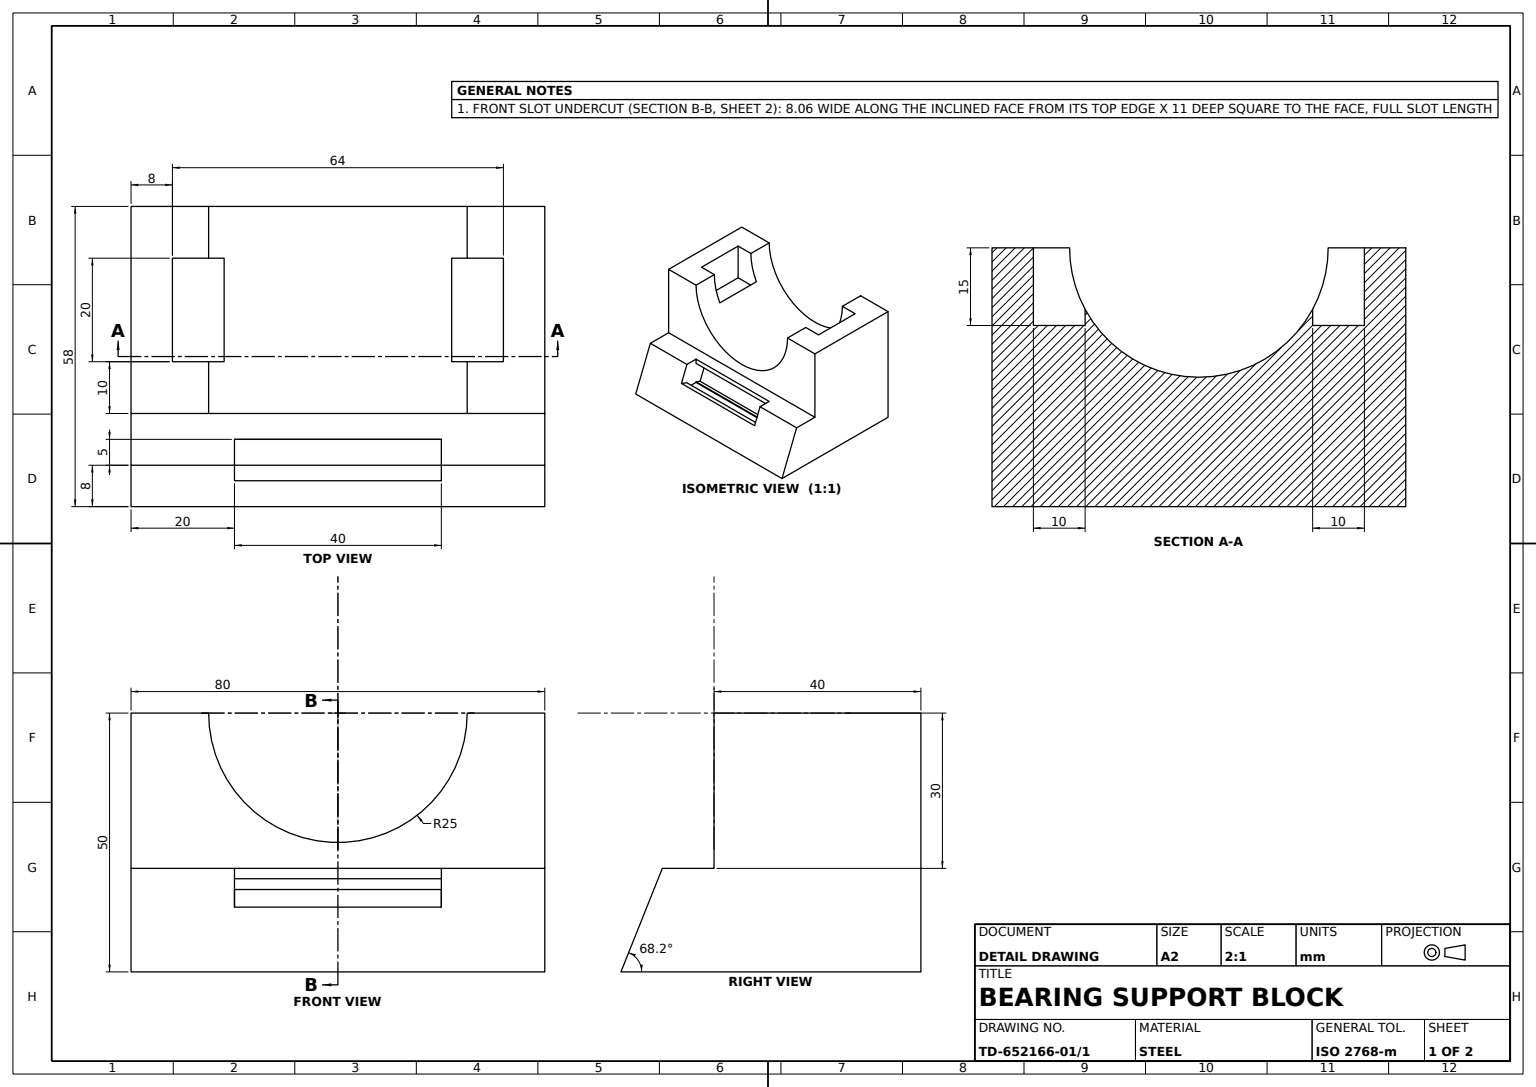
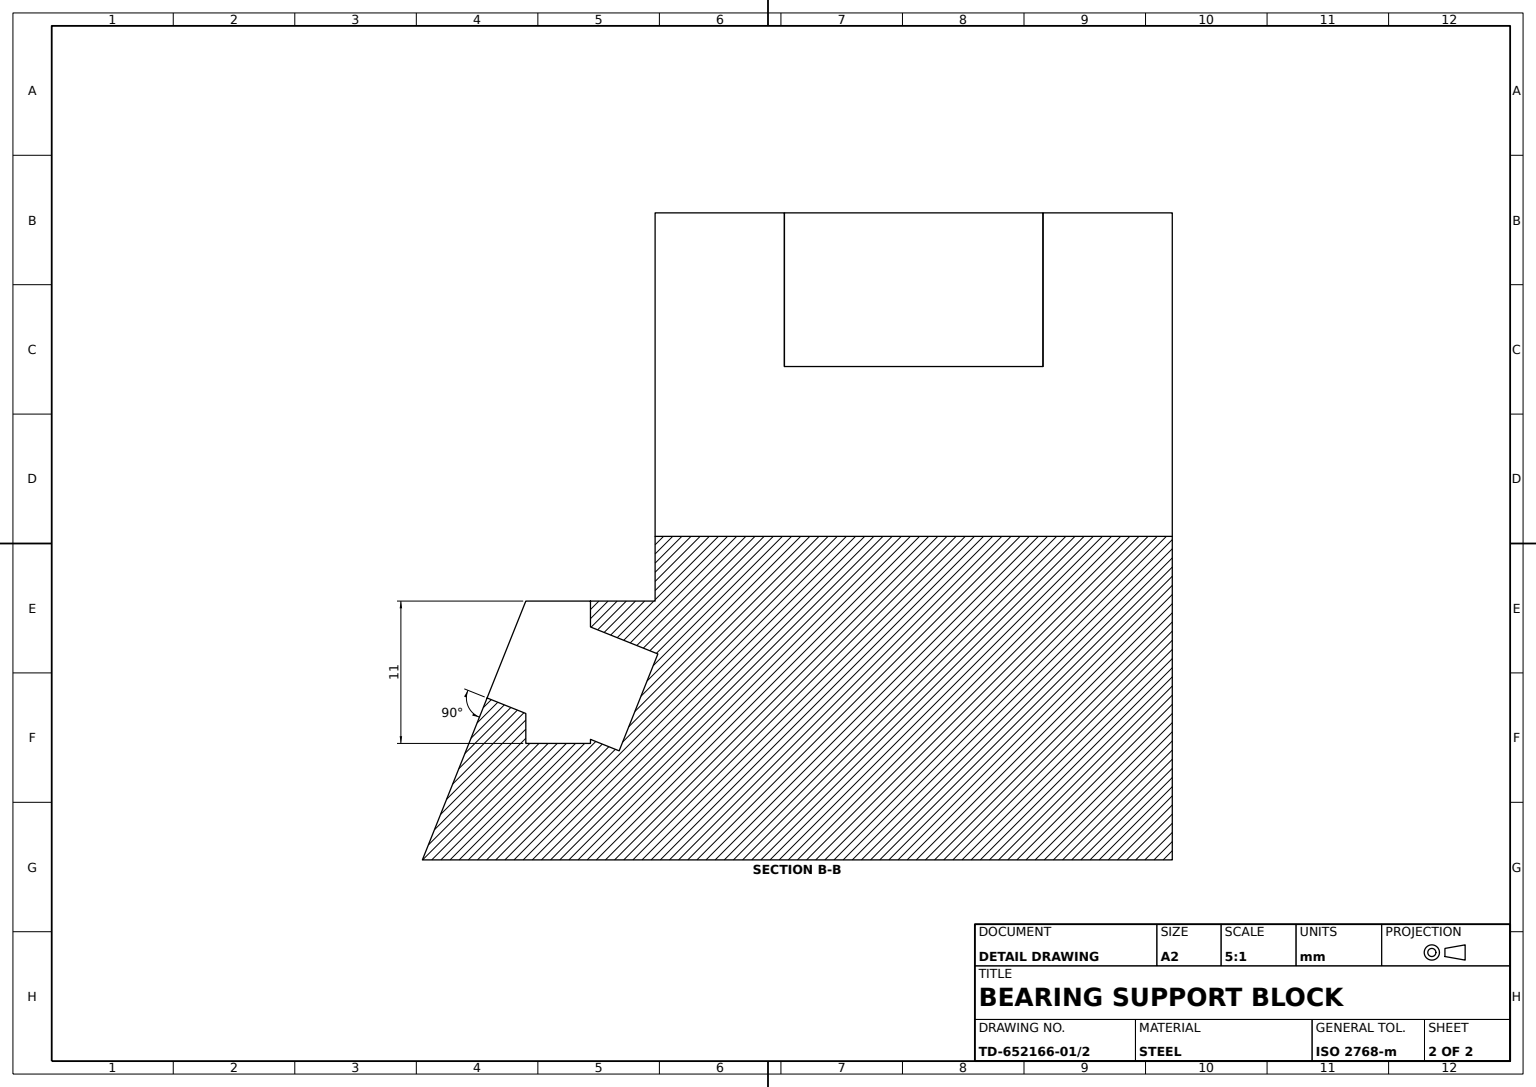
from build123d import *

# Parameters (mm, degrees)
BASE_BLOCK_DEPTH             = 80
UPRIGHT_NOTCHES_SKETCH_W     = 20
UPRIGHT_NOTCHES_SKETCH_H     = 10
UPRIGHT_TOP_NOTCHES_DEPTH    = 15
SADDLE_BORE_SKETCH_R         = 25
SADDLE_BORE_50_DEPTH         = 103.46950766
FRONT_SLOPE_CUT_DEPTH        = 111.742945599
FRONT_SLOT_SKETCH_W          = 5
FRONT_SLOT_SKETCH_H          = 40
FRONT_SLOT_40X5_DEPTH        = 11
FRONT_SLOT_UNDERCUT_SKETCH_W = 40
FRONT_SLOT_UNDERCUT_SKETCH_H = 8.064305279
FRONT_SLOT_UNDERCUT_DEPTH    = 11


with BuildPart() as part:
    # Base Profile Sketch → Base Block (new body)
    with BuildSketch(Plane.XY):
        Polygon((0, 0), (0, 50), (40, 50), (40, 20), (58, 20), (58, 0), align=None)
    extrude(amount=BASE_BLOCK_DEPTH)

    # Upright Notches Sketch → Upright Top Notches (cut)
    with BuildSketch(Plane(origin=(0, 50, 0), x_dir=(1, 0, 0), z_dir=(0, 1, 0))):
        with Locations((20, -13)):
            Rectangle(UPRIGHT_NOTCHES_SKETCH_W, UPRIGHT_NOTCHES_SKETCH_H)
        with Locations((20, -67)):
            Rectangle(UPRIGHT_NOTCHES_SKETCH_W, UPRIGHT_NOTCHES_SKETCH_H)
    extrude(amount=-UPRIGHT_TOP_NOTCHES_DEPTH, mode=Mode.SUBTRACT)

    # Saddle Bore Sketch → Saddle Bore Ø50 (cut, through all)
    with BuildSketch(Plane(origin=(40, 0, 0), x_dir=(0, 0, -1), z_dir=(1, 0, 0))):
        with Locations((-40, 50)):
            Circle(SADDLE_BORE_SKETCH_R)
    extrude(amount=-SADDLE_BORE_50_DEPTH, mode=Mode.SUBTRACT)

    # Front Slope Sketch → Front Slope Cut (cut, through all)
    with BuildSketch(Plane.XY.offset(80)):
        Polygon((50, 20), (58, 20), (58, 0), align=None)
    extrude(amount=-FRONT_SLOPE_CUT_DEPTH, mode=Mode.SUBTRACT)

    # Front Slot Sketch → Front Slot 40x5 (cut)
    with BuildSketch(Plane(origin=(0, 20, 0), x_dir=(1, 0, 0), z_dir=(0, 1, 0))):
        with Locations((47.5, -40)):
            Rectangle(FRONT_SLOT_SKETCH_W, FRONT_SLOT_SKETCH_H)
    extrude(amount=-FRONT_SLOT_40X5_DEPTH, mode=Mode.SUBTRACT)

    # Front Slot Undercut Sketch → Front Slot Undercut (cut)
    with BuildSketch(Plane(origin=(50, 20, 0), x_dir=(0, 0, -1), z_dir=(0.9284766908852593, 0.3713906763541041, 0))):
        with Locations((-40, -4.03215264)):
            Rectangle(FRONT_SLOT_UNDERCUT_SKETCH_W, FRONT_SLOT_UNDERCUT_SKETCH_H)
    extrude(amount=-FRONT_SLOT_UNDERCUT_DEPTH, mode=Mode.SUBTRACT)


solid = part.part
